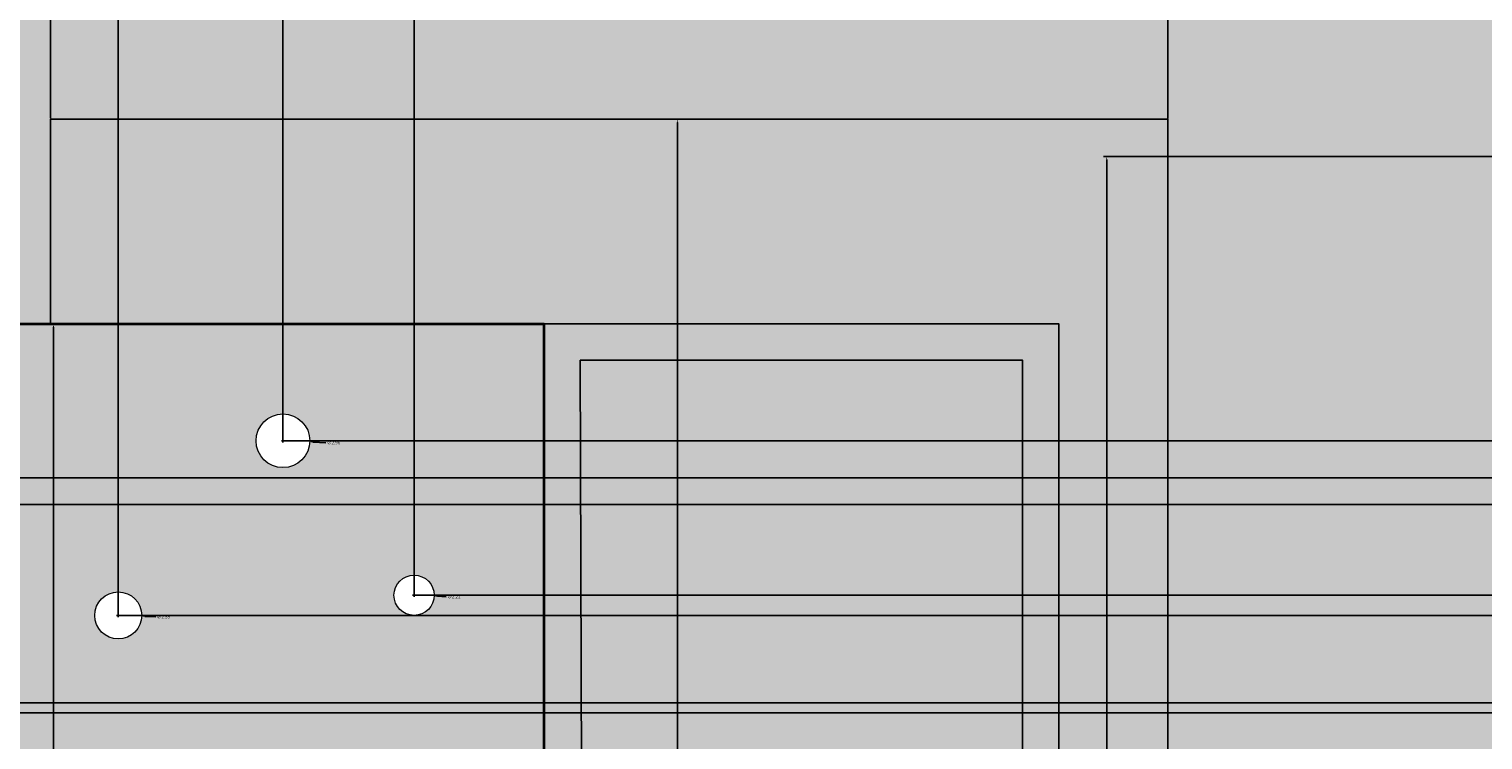
# Model space of a CAD drawing. Units: inches. Extents: x 73 to 607, y 92 to 651.
# Tile 5 of 18: x 368 to 448, y 224 to 264. Entities that reach past the tile are written whole.
import ezdxf

# ---------------------------------------------------------------- set-up
doc = ezdxf.new("R2010")
doc.units = ezdxf.units.IN
doc.header["$MEASUREMENT"] = 0
for name, color, linetype, lineweight in [('A-ANNO-DIMS', 2, 'Continuous', 18), ('A-ELEV', 7, 'Continuous', 35), ('A-ELEV-PANL', 7, 'Continuous', 18), ('A-ELEV-PATT-BKGD', 252, 'Continuous', 13), ('A-ELEV-PATT-FRAM', 38, 'Continuous', 13), ('A-ELEV-PATT-SHAD', 8, 'Continuous', 13), ('A-ELEV-PATT-WALL', 254, 'Continuous', 13), ('A-ELEV-PATT-WOOD', 32, 'Continuous', 13), ('A-GLAZ', 4, 'Continuous', 25), ('A-GLAZ-PATT', 7, 'Continuous', 13)]:
    doc.layers.add(name, color=color, linetype=linetype, lineweight=lineweight)
doc.styles.get("Standard").update_dxf_attribs({"font": 'arial.ttf'})
doc.dimstyles.get("Standard").update_dxf_attribs({"dimtxt": 0.18, "dimasz": 0.18, "dimexe": 0.18, "dimexo": 0.0625, "dimgap": 0.09, "dimtad": 0, "dimtih": 1, "dimtoh": 1, "dimdec": 4, "dimzin": 0, "dimdsep": 46, "dimtxsty": 'Standard', "dimcen": 0.09, "dimadec": 0, "dimazin": 0, "dimtfac": 1, "dimtdec": 4, "dimtofl": 0, "dimtmove": 0, "dimatfit": 3, "dimfxl": 1, "dimtolj": 1, "dimtzin": 0, "dimarcsym": 0})

# ---------------------------------------------------------------- blocks, each defined once
blk = doc.blocks.new('*D17')
at = {"layer": 'A-ANNO-DIMS', "color": 0, "lineweight": -2, "transparency": 16777216}
for p, q in [((580.161, 262.302), (607.278, 262.302)), ((607.098, 262.122), (607.098, 224.164)), ((607.098, 185.842), (607.098, 223.8)), ((431.133, 185.662), (607.278, 185.662))]:
    blk.add_line(p, q, dxfattribs=at)
at = {"layer": 'A-ANNO-DIMS', "color": 0, "transparency": 16777216}
for points in [[(607.068, 262.122), (607.128, 262.122), (607.098, 262.302)], [(607.068, 185.842), (607.128, 185.842), (607.098, 185.662)]]:
    blk.add_solid(points, dxfattribs=at)
at = {"layer": 'Defpoints', "color": 0, "transparency": 16777216}
for p in [(580.098, 262.302), (607.098, 262.302), (431.07, 185.662)]:
    blk.add_point(p, dxfattribs=at)
at = {"layer": 'A-ANNO-DIMS', "color": 0, "transparency": 16777216, "insert": (607.098, 223.982), "char_height": 0.18, "attachment_point": 5}
blk.add_mtext('\\A1;76.64', dxfattribs=at)
blk = doc.blocks.new('*D36')
at = {"layer": 'A-ANNO-DIMS', "color": 0, "lineweight": -2, "transparency": 16777216}
for p, q in [((396.63, 247.405), (369.512, 247.405)), ((369.692, 247.225), (369.692, 221.153)), ((369.692, 194.717), (369.692, 220.789)), ((396.63, 194.537), (369.512, 194.537))]:
    blk.add_line(p, q, dxfattribs=at)
at = {"layer": 'A-ANNO-DIMS', "color": 0, "transparency": 16777216}
for points in [[(369.662, 247.225), (369.722, 247.225), (369.692, 247.405)], [(369.662, 194.717), (369.722, 194.717), (369.692, 194.537)]]:
    blk.add_solid(points, dxfattribs=at)
at = {"layer": 'Defpoints', "color": 0, "transparency": 16777216}
for p in [(369.692, 247.405), (396.692, 247.405), (396.692, 194.537)]:
    blk.add_point(p, dxfattribs=at)
at = {"layer": 'A-ANNO-DIMS', "color": 0, "transparency": 16777216, "insert": (369.692, 220.971), "char_height": 0.18, "attachment_point": 5}
blk.add_mtext('\\A1;52.87', dxfattribs=at)
blk = doc.blocks.new('*D37')
at = {"layer": 'A-ANNO-DIMS', "color": 0, "lineweight": -2, "transparency": 16777216}
for p, q in [((369.534, 258.754), (369.534, 285.871)), ((369.714, 285.691), (399.908, 285.691)), ((430.89, 285.691), (400.696, 285.691)), ((431.07, 258.754), (431.07, 285.871))]:
    blk.add_line(p, q, dxfattribs=at)
at = {"layer": 'A-ANNO-DIMS', "color": 0, "transparency": 16777216}
for points in [[(369.714, 285.721), (369.714, 285.661), (369.534, 285.691)], [(430.89, 285.721), (430.89, 285.661), (431.07, 285.691)]]:
    blk.add_solid(points, dxfattribs=at)
at = {"layer": 'Defpoints', "color": 0, "transparency": 16777216}
for p in [(431.07, 285.691), (369.534, 258.691), (431.07, 258.691)]:
    blk.add_point(p, dxfattribs=at)
at = {"layer": 'A-ANNO-DIMS', "color": 0, "transparency": 16777216, "insert": (400.302, 285.691), "char_height": 0.18, "attachment_point": 5}
blk.add_mtext('\\A1;61.54', dxfattribs=at)
blk = doc.blocks.new('*D38')
at = {"layer": 'A-ANNO-DIMS', "color": 0, "lineweight": -2, "transparency": 16777216}
for p, q in [((431.008, 258.691), (403.89, 258.691)), ((404.07, 258.511), (404.07, 222.359)), ((404.07, 185.842), (404.07, 221.995)), ((431.008, 185.662), (403.89, 185.662))]:
    blk.add_line(p, q, dxfattribs=at)
at = {"layer": 'A-ANNO-DIMS', "color": 0, "transparency": 16777216}
for points in [[(404.04, 258.511), (404.1, 258.511), (404.07, 258.691)], [(404.04, 185.842), (404.1, 185.842), (404.07, 185.662)]]:
    blk.add_solid(points, dxfattribs=at)
at = {"layer": 'Defpoints', "color": 0, "transparency": 16777216}
for p in [(404.07, 258.691), (431.07, 258.691), (431.07, 185.662)]:
    blk.add_point(p, dxfattribs=at)
at = {"layer": 'A-ANNO-DIMS', "color": 0, "transparency": 16777216, "insert": (404.07, 222.177), "char_height": 0.18, "attachment_point": 5}
blk.add_mtext('\\A1;73.03', dxfattribs=at)
blk = doc.blocks.new('*D40')
at = {"layer": 'A-ANNO-DIMS', "color": 0, "lineweight": -2, "transparency": 16777216}
for p, q in [((454.642, 256.632), (427.525, 256.632)), ((427.705, 256.452), (427.705, 215.899)), ((427.705, 174.982), (427.705, 215.535)), ((454.642, 174.802), (427.525, 174.802))]:
    blk.add_line(p, q, dxfattribs=at)
at = {"layer": 'A-ANNO-DIMS', "color": 0, "transparency": 16777216}
for points in [[(427.675, 256.452), (427.735, 256.452), (427.705, 256.632)], [(427.675, 174.982), (427.735, 174.982), (427.705, 174.802)]]:
    blk.add_solid(points, dxfattribs=at)
at = {"layer": 'Defpoints', "color": 0, "transparency": 16777216}
for p in [(427.705, 256.632), (454.705, 256.632), (454.705, 174.802)]:
    blk.add_point(p, dxfattribs=at)
at = {"layer": 'A-ANNO-DIMS', "color": 0, "transparency": 16777216, "insert": (427.705, 215.717), "char_height": 0.18, "attachment_point": 5}
blk.add_mtext('\\A1;81.83', dxfattribs=at)
blk = doc.blocks.new('*D83')
at = {"layer": 'A-ANNO-DIMS', "color": 0, "lineweight": -2, "transparency": 16777216}
for p, q in [((360.849, 238.997), (360.849, 650.981)), ((361.029, 650.801), (366.597, 650.801)), ((373.077, 650.801), (367.508, 650.801)), ((373.257, 231.411), (373.257, 650.981))]:
    blk.add_line(p, q, dxfattribs=at)
at = {"layer": 'A-ANNO-DIMS', "color": 0, "transparency": 16777216}
for points in [[(361.029, 650.831), (361.029, 650.771), (360.849, 650.801)], [(373.077, 650.831), (373.077, 650.771), (373.257, 650.801)]]:
    blk.add_solid(points, dxfattribs=at)
at = {"layer": 'Defpoints', "color": 0, "transparency": 16777216}
for p in [(373.257, 650.801), (360.849, 238.935), (373.257, 231.348)]:
    blk.add_point(p, dxfattribs=at)
at = {"layer": 'A-ANNO-DIMS', "color": 0, "transparency": 16777216, "insert": (367.053, 650.801), "char_height": 0.18, "attachment_point": 5}
blk.add_mtext('\\A1;12.408', dxfattribs=at)
blk = doc.blocks.new('*D84')
at = {"layer": 'A-ANNO-DIMS', "color": 0, "lineweight": -2, "transparency": 16777216}
for p, q in [((373.257, 231.411), (373.257, 650.981)), ((373.437, 650.801), (377.4, 650.801)), ((382.151, 650.801), (378.187, 650.801)), ((382.331, 241.033), (382.331, 650.981))]:
    blk.add_line(p, q, dxfattribs=at)
at = {"layer": 'A-ANNO-DIMS', "color": 0, "transparency": 16777216}
for points in [[(373.437, 650.831), (373.437, 650.771), (373.257, 650.801)], [(382.151, 650.831), (382.151, 650.771), (382.331, 650.801)]]:
    blk.add_solid(points, dxfattribs=at)
at = {"layer": 'Defpoints', "color": 0, "transparency": 16777216}
for p in [(382.331, 650.801), (382.331, 240.97), (373.257, 231.348)]:
    blk.add_point(p, dxfattribs=at)
at = {"layer": 'A-ANNO-DIMS', "color": 0, "transparency": 16777216, "insert": (377.794, 650.801), "char_height": 0.18, "attachment_point": 5}
blk.add_mtext('\\A1;9.074', dxfattribs=at)
blk = doc.blocks.new('*D85')
at = {"layer": 'A-ANNO-DIMS', "color": 0, "lineweight": -2, "transparency": 16777216}
for p, q in [((382.331, 241.033), (382.331, 650.981)), ((382.511, 650.801), (385.55, 650.801)), ((389.373, 650.801), (386.334, 650.801)), ((389.553, 232.521), (389.553, 650.981))]:
    blk.add_line(p, q, dxfattribs=at)
at = {"layer": 'A-ANNO-DIMS', "color": 0, "transparency": 16777216}
for points in [[(382.511, 650.831), (382.511, 650.771), (382.331, 650.801)], [(389.373, 650.831), (389.373, 650.771), (389.553, 650.801)]]:
    blk.add_solid(points, dxfattribs=at)
at = {"layer": 'Defpoints', "color": 0, "transparency": 16777216}
for p in [(389.553, 650.801), (382.331, 240.97), (389.553, 232.458)]:
    blk.add_point(p, dxfattribs=at)
at = {"layer": 'A-ANNO-DIMS', "color": 0, "transparency": 16777216, "insert": (385.942, 650.801), "char_height": 0.18, "attachment_point": 5}
blk.add_mtext('\\A1;7.222', dxfattribs=at)
blk = doc.blocks.new('*D93')
at = {"layer": 'A-ANNO-DIMS', "color": 0, "lineweight": -2, "transparency": 16777216}
for p, q in [((349.059, 237.455), (607.278, 237.455)), ((607.098, 237.275), (607.098, 232.178)), ((607.098, 226.717), (607.098, 231.814)), ((349.059, 226.537), (607.278, 226.537))]:
    blk.add_line(p, q, dxfattribs=at)
at = {"layer": 'A-ANNO-DIMS', "color": 0, "transparency": 16777216}
for points in [[(607.068, 237.275), (607.128, 237.275), (607.098, 237.455)], [(607.068, 226.717), (607.128, 226.717), (607.098, 226.537)]]:
    blk.add_solid(points, dxfattribs=at)
at = {"layer": 'Defpoints', "color": 0, "transparency": 16777216}
for p in [(348.997, 237.455), (348.997, 226.537), (607.098, 226.537)]:
    blk.add_point(p, dxfattribs=at)
at = {"layer": 'A-ANNO-DIMS', "color": 0, "transparency": 16777216, "insert": (607.098, 231.996), "char_height": 0.18, "attachment_point": 5}
blk.add_mtext('\\A1;10.917', dxfattribs=at)
blk = doc.blocks.new('*D95')
at = {"layer": 'A-ANNO-DIMS', "color": 0, "lineweight": -2, "transparency": 16777216}
for p, q in [((363.874, 225.982), (607.278, 225.982)), ((607.098, 225.802), (607.098, 212.749)), ((607.098, 199.331), (607.098, 212.385)), ((363.319, 199.151), (607.278, 199.151))]:
    blk.add_line(p, q, dxfattribs=at)
at = {"layer": 'A-ANNO-DIMS', "color": 0, "transparency": 16777216}
for points in [[(607.068, 225.802), (607.128, 225.802), (607.098, 225.982)], [(607.068, 199.331), (607.128, 199.331), (607.098, 199.151)]]:
    blk.add_solid(points, dxfattribs=at)
at = {"layer": 'Defpoints', "color": 0, "transparency": 16777216}
for p in [(363.812, 225.982), (607.098, 225.982), (363.256, 199.151)]:
    blk.add_point(p, dxfattribs=at)
at = {"layer": 'A-ANNO-DIMS', "color": 0, "transparency": 16777216, "insert": (607.098, 212.567), "char_height": 0.18, "attachment_point": 5}
blk.add_mtext('\\A1;26.83', dxfattribs=at)
blk = doc.blocks.new('*D96')
at = {"layer": 'A-ANNO-DIMS', "color": 0, "lineweight": -2, "transparency": 16777216}
for p, q in [((360.911, 238.935), (607.278, 238.935)), ((607.098, 238.755), (607.098, 232.64)), ((607.098, 226.162), (607.098, 232.276)), ((363.874, 225.982), (607.278, 225.982))]:
    blk.add_line(p, q, dxfattribs=at)
at = {"layer": 'A-ANNO-DIMS', "color": 0, "transparency": 16777216}
for points in [[(607.068, 238.755), (607.128, 238.755), (607.098, 238.935)], [(607.068, 226.162), (607.128, 226.162), (607.098, 225.982)]]:
    blk.add_solid(points, dxfattribs=at)
at = {"layer": 'Defpoints', "color": 0, "transparency": 16777216}
for p in [(360.849, 238.935), (607.098, 238.935), (363.812, 225.982)]:
    blk.add_point(p, dxfattribs=at)
at = {"layer": 'A-ANNO-DIMS', "color": 0, "transparency": 16777216, "insert": (607.098, 232.458), "char_height": 0.18, "attachment_point": 5}
blk.add_mtext('\\A1;12.953', dxfattribs=at)
blk = doc.blocks.new('*D99')
at = {"layer": 'A-ANNO-DIMS', "color": 0, "lineweight": -2, "transparency": 16777216}
for p, q in [((373.319, 231.348), (607.278, 231.348)), ((607.098, 231.168), (607.098, 220.428)), ((607.098, 209.323), (607.098, 220.064)), ((377.023, 209.143), (607.278, 209.143))]:
    blk.add_line(p, q, dxfattribs=at)
at = {"layer": 'A-ANNO-DIMS', "color": 0, "transparency": 16777216}
for points in [[(607.068, 231.168), (607.128, 231.168), (607.098, 231.348)], [(607.068, 209.323), (607.128, 209.323), (607.098, 209.143)]]:
    blk.add_solid(points, dxfattribs=at)
at = {"layer": 'Defpoints', "color": 0, "transparency": 16777216}
for p in [(373.257, 231.348), (607.098, 231.348), (376.96, 209.143)]:
    blk.add_point(p, dxfattribs=at)
at = {"layer": 'A-ANNO-DIMS', "color": 0, "transparency": 16777216, "insert": (607.098, 220.246), "char_height": 0.18, "attachment_point": 5}
blk.add_mtext('\\A1;22.205', dxfattribs=at)
blk = doc.blocks.new('*D101')
at = {"layer": 'A-ANNO-DIMS', "color": 0, "lineweight": -2, "transparency": 16777216}
for p, q in [((382.393, 240.97), (607.278, 240.97)), ((607.098, 240.79), (607.098, 231.715)), ((607.098, 222.276), (607.098, 231.351)), ((382.949, 222.096), (607.278, 222.096))]:
    blk.add_line(p, q, dxfattribs=at)
at = {"layer": 'A-ANNO-DIMS', "color": 0, "transparency": 16777216}
for points in [[(607.068, 240.79), (607.128, 240.79), (607.098, 240.97)], [(607.068, 222.276), (607.128, 222.276), (607.098, 222.096)]]:
    blk.add_solid(points, dxfattribs=at)
at = {"layer": 'Defpoints', "color": 0, "transparency": 16777216}
for p in [(382.331, 240.97), (607.098, 240.97), (382.886, 222.096)]:
    blk.add_point(p, dxfattribs=at)
at = {"layer": 'A-ANNO-DIMS', "color": 0, "transparency": 16777216, "insert": (607.098, 231.533), "char_height": 0.18, "attachment_point": 5}
blk.add_mtext('\\A1;18.874', dxfattribs=at)
blk = doc.blocks.new('*D102')
at = {"layer": 'A-ANNO-DIMS', "color": 0, "lineweight": -2, "transparency": 16777216}
for p, q in [((382.393, 240.97), (607.278, 240.97)), ((607.098, 240.79), (607.098, 236.896)), ((607.098, 232.638), (607.098, 236.532)), ((389.616, 232.458), (607.278, 232.458))]:
    blk.add_line(p, q, dxfattribs=at)
at = {"layer": 'A-ANNO-DIMS', "color": 0, "transparency": 16777216}
for points in [[(607.068, 240.79), (607.128, 240.79), (607.098, 240.97)], [(607.068, 232.638), (607.128, 232.638), (607.098, 232.458)]]:
    blk.add_solid(points, dxfattribs=at)
at = {"layer": 'Defpoints', "color": 0, "transparency": 16777216}
for p in [(382.331, 240.97), (389.553, 232.458), (607.098, 232.458)]:
    blk.add_point(p, dxfattribs=at)
at = {"layer": 'A-ANNO-DIMS', "color": 0, "transparency": 16777216, "insert": (607.098, 236.714), "char_height": 0.18, "attachment_point": 5}
blk.add_mtext('\\A1;8.512', dxfattribs=at)
blk = doc.blocks.new('*D144')
at = {"layer": 'A-ANNO-DIMS', "color": 0, "lineweight": -2, "transparency": 16777216}
for p, q in [((382.331, 240.88), (382.331, 241.06)), ((382.241, 240.97), (382.421, 240.97)), ((384.697, 240.864), (383.989, 240.896))]:
    blk.add_line(p, q, dxfattribs=at)
at = {"layer": 'A-ANNO-DIMS', "color": 0, "transparency": 16777216}
blk.add_solid([(383.991, 240.925), (383.988, 240.866), (383.81, 240.904)], dxfattribs=at)
at = {"layer": 'Defpoints', "color": 0, "transparency": 16777216}
for p in [(380.852, 241.037), (383.81, 240.904)]:
    blk.add_point(p, dxfattribs=at)
at = {"layer": 'A-ANNO-DIMS', "color": 0, "transparency": 16777216, "insert": (385.119, 240.864), "char_height": 0.18, "attachment_point": 5}
blk.add_mtext('\\A1;∅2.96', dxfattribs=at)
blk = doc.blocks.new('*D145')
at = {"layer": 'A-ANNO-DIMS', "color": 0, "lineweight": -2, "transparency": 16777216}
for p, q in [((373.257, 231.258), (373.257, 231.438)), ((373.167, 231.348), (373.347, 231.348)), ((375.328, 231.273), (374.731, 231.295))]:
    blk.add_line(p, q, dxfattribs=at)
at = {"layer": 'A-ANNO-DIMS', "color": 0, "transparency": 16777216}
blk.add_solid([(374.732, 231.325), (374.73, 231.265), (374.551, 231.301)], dxfattribs=at)
at = {"layer": 'Defpoints', "color": 0, "transparency": 16777216}
for p in [(371.962, 231.395), (374.551, 231.301)]:
    blk.add_point(p, dxfattribs=at)
at = {"layer": 'A-ANNO-DIMS', "color": 0, "transparency": 16777216, "insert": (375.75, 231.273), "char_height": 0.18, "attachment_point": 5}
blk.add_mtext('\\A1;∅2.59', dxfattribs=at)
blk = doc.blocks.new('*D146')
at = {"layer": 'A-ANNO-DIMS', "color": 0, "lineweight": -2, "transparency": 16777216}
for p, q in [((389.463, 232.458), (389.643, 232.458)), ((389.553, 232.368), (389.553, 232.548)), ((391.328, 232.376), (390.842, 232.399))]:
    blk.add_line(p, q, dxfattribs=at)
at = {"layer": 'A-ANNO-DIMS', "color": 0, "transparency": 16777216}
blk.add_solid([(390.843, 232.428), (390.841, 232.369), (390.662, 232.407)], dxfattribs=at)
at = {"layer": 'Defpoints', "color": 0, "transparency": 16777216}
for p in [(388.444, 232.51), (390.662, 232.407)]:
    blk.add_point(p, dxfattribs=at)
at = {"layer": 'A-ANNO-DIMS', "color": 0, "transparency": 16777216, "insert": (391.748, 232.376), "char_height": 0.18, "attachment_point": 5}
blk.add_mtext('\\A1;∅2.22', dxfattribs=at)

msp = doc.modelspace()

# ---------------------------------------------------------------- hatches: boundary and pattern name
at = {"layer": 'A-ELEV-PATT-BKGD'}
h = msp.add_hatch(color=256, dxfattribs=at)
h.dxf.hatch_style = 1
h.paths.add_polyline_path([(321.3008, 479.2042), (312.3008, 479.2042), (312.3008, 478.7576), (312.3008, 412.636), (321.3008, 412.636)])
h.paths.add_polyline_path([(312.3008, 504.7576), (256.4726, 504.7576), (256.4726, 503.4576), (312.3008, 503.4576)], flags=17)
h.paths.add_polyline_path([(321.3008, 543.1576), (321.3008, 552.1576), (320.3257, 552.1576), (312.3008, 552.1576), (256.4726, 552.1576), (256.4726, 543.1576), (312.3008, 543.1576), (312.3008, 479.2042), (321.3008, 479.2042)])
h.paths.add_polyline_path([(451.5214, 412.636), (256.4726, 412.636), (256.4726, 403.636), (442.5214, 403.636), (442.5214, 320.2042), (206.1343, 320.2042), (206.1343, 320.9135), (206.1343, 403.636), (256.4726, 403.636), (256.4726, 412.636), (201.6343, 412.636), (201.6343, 320.9135), (201.6343, 320.2042), (201.6343, 311.2042), (256.4726, 311.2042), (451.5214, 311.2042)])
h.paths.add_polyline_path([(431.07, 258.6914), (369.5339, 258.6914), (369.5339, 247.4054), (396.692, 247.4054), (425.07, 247.4054), (425.07, 194.7312), (396.692, 194.6197), (396.692, 194.5366), (369.5339, 194.5366), (369.5339, 185.6619), (431.07, 185.6619)])
h.paths.add_polyline_path([(580.0983, 262.3024), (451.5214, 262.3024), (451.5214, 143.2042), (580.0983, 143.2042)])
h.paths.add_polyline_path([(454.7049, 174.802), (454.7049, 256.6321), (577.9249, 256.6321), (577.9249, 174.802)], flags=16)
h.paths.add_polyline_path([(465.9716, 191.1416, -1), (473.7874, 191.1416, -1)], flags=0)
h.paths.add_polyline_path([(490.5373, 181.6586, -1), (494.9999, 181.6586, -1)], flags=0)
h.paths.add_polyline_path([(476.2996, 209.8287, -1), (500.5844, 209.8287, -1)], flags=0)
h.paths.add_polyline_path([(505.3326, 194.7675, -1), (512.5843, 194.7675, -1)], flags=0)
h.paths.add_polyline_path([(520.9613, 186.679, -1), (526.544, 186.679, -1)], flags=0)
h.paths.add_polyline_path([(466.8103, 225.7267, -1), (470.1573, 225.7267, -1)], flags=0)
h.paths.add_polyline_path([(527.1059, 203.6926, -1), (536.0311, 203.6926, -1)], flags=0)
h.paths.add_polyline_path([(504.775, 232.6995, -1), (513.7002, 232.6995, -1)], flags=0)
h.paths.add_polyline_path([(546.9241, 183.611, -1), (554.7336, 183.611, -1)], flags=0)
h.paths.add_polyline_path([(459.5544, 243.856, -1), (466.8061, 243.856, -1)], flags=0)
h.paths.add_polyline_path([(476.3045, 246.924, -1), (488.5767, 246.924, -1)], flags=0)
h.paths.add_polyline_path([(529.9044, 226.8424, -1), (556.68, 226.8424, -1)], flags=0)
h.paths.add_polyline_path([(554.1814, 203.9716, -1), (561.4331, 203.9716, -1)], flags=0)
h.paths.add_polyline_path([(567.8561, 193.3729, -1), (570.6475, 193.3729, -1)], flags=0)
h.paths.add_polyline_path([(522.3584, 250.271, -1), (525.7053, 250.271, -1)], flags=0)
h.paths.add_polyline_path([(561.9965, 245.2506, -1), (567.5748, 245.2506, -1)], flags=0)
h.paths.add_polyline_path([(347.8686, 194.5366), (341.8686, 194.5366), (341.8686, 194.5452), (314.0144, 194.5452), (314.0144, 188.5452), (347.8686, 188.5452)])
h.paths.add_polyline_path([(347.8686, 253.4054), (314.0144, 253.4054), (314.0144, 247.4054), (341.8686, 247.4054), (347.8686, 247.4054)])
h.paths.add_polyline_path([(304.3559, 253.4054), (298.3559, 253.4054), (298.3559, 188.5452), (304.3559, 188.5452)])
h.paths.add_polyline_path([(450.6603, 552.1576), (369.9727, 552.1576), (369.9727, 479.2042), (374.4727, 479.2042), (374.4727, 547.6576), (446.1603, 547.6576), (446.1603, 479.2042), (450.6603, 479.2042)])
h.paths.add_polyline_path([(374.4727, 479.2042), (369.9727, 479.2042), (369.9727, 465.0632), (374.4727, 465.0632)])
h.paths.add_polyline_path([(450.6603, 479.2042), (446.1603, 479.2042), (446.1603, 465.0632), (450.6603, 465.0632)])
h.paths.add_polyline_path([(256.4726, 281.6039), (109.0983, 281.6039), (100.0983, 281.6039), (100.0983, 167.2042), (100.0983, 143.2042), (109.0983, 143.2042), (109.0983, 167.2042), (109.0983, 272.6039), (256.4726, 272.6039)])
at = {"layer": 'A-ELEV-PATT-FRAM'}
h = msp.add_hatch(color=256, dxfattribs=at)
h.dxf.hatch_style = 1
h.paths.add_polyline_path([(433.025, 403.636), (409.515, 403.636), (409.515, 342.1009), (411.515, 342.1009), (411.515, 401.636), (431.025, 401.636), (431.025, 342.1009), (433.025, 342.1009)])
h.paths.add_polyline_path([(433.025, 341.1009), (431.025, 341.1009), (431.025, 340.0025), (411.515, 340.0025), (411.515, 341.1009), (409.515, 341.1009), (409.515, 338.0025), (433.025, 338.0025)])
h.paths.add_polyline_path([(425.07, 247.4054), (396.692, 247.4054), (396.692, 194.6197), (425.07, 194.7312)])
h.paths.add_polyline_path([(423.07, 245.4054), (423.07, 196.7234), (398.8836, 196.6284), (398.692, 245.4054)], flags=16)
h.paths.add_polyline_path([(341.8686, 247.4054), (314.0144, 247.4054), (314.0144, 245.4054), (339.8686, 245.4054), (339.8686, 196.5452), (314.0144, 196.5452), (314.0144, 194.5452), (341.8686, 194.5452)])
h.paths.add_polyline_path([(372.3213, 383.1812), (350.3213, 383.1812), (350.3213, 342.1009), (372.3213, 342.1009)], flags=16)
h.paths.add_polyline_path([(376.3213, 389.1812), (346.3213, 389.1812), (346.3213, 342.1009), (350.3213, 342.1009), (350.3213, 383.1812), (372.3213, 383.1812), (372.3213, 342.1009), (376.3213, 342.1009)], flags=17)
h.paths.add_polyline_path([(375.3213, 362.2042, -1), (373.3213, 362.2042, -1)], flags=16)
h.paths.add_polyline_path([(379.3213, 392.2042), (343.3213, 392.2042), (343.3213, 342.1009), (346.3213, 342.1009), (346.3213, 389.1812), (376.3213, 389.1812), (376.3213, 342.1009), (379.3213, 342.1009)])
h.paths.add_polyline_path([(350.3213, 341.1009), (346.3213, 341.1009), (346.3213, 338.0025), (350.3213, 338.0025)])
h.paths.add_polyline_path([(346.3213, 341.1009), (343.3213, 341.1009), (343.3213, 338.0025), (346.3213, 338.0025)])
h.paths.add_polyline_path([(346.3213, 337.0025), (343.3213, 337.0025), (343.3213, 332.9397), (346.3213, 332.9397)])
h.paths.add_polyline_path([(350.3213, 337.0025), (346.3213, 337.0025), (346.3213, 332.9397), (350.3213, 332.9397)])
h.paths.add_polyline_path([(350.3213, 331.9397), (346.3213, 331.9397), (346.3213, 320.2042), (376.3213, 320.2042), (376.3213, 331.9397), (372.3213, 331.9397), (372.3213, 326.2042), (350.3213, 326.2042)])
h.paths.add_polyline_path([(372.3213, 337.0025), (350.3213, 337.0025), (350.3213, 332.9397), (372.3213, 332.9397)])
h.paths.add_polyline_path([(372.3213, 341.1009), (350.3213, 341.1009), (350.3213, 338.0025), (372.3213, 338.0025)])
h.paths.add_polyline_path([(376.3213, 341.1009), (372.3213, 341.1009), (372.3213, 338.0025), (376.3213, 338.0025)])
h.paths.add_polyline_path([(376.3213, 337.0025), (372.3213, 337.0025), (372.3213, 332.9397), (376.3213, 332.9397)])
h.paths.add_polyline_path([(379.3213, 341.1009), (376.3213, 341.1009), (376.3213, 338.0025), (379.3213, 338.0025)])
h.paths.add_polyline_path([(379.3213, 337.0025), (376.3213, 337.0025), (376.3213, 332.9397), (379.3213, 332.9397)])
h.paths.add_polyline_path([(379.3213, 331.9397), (376.3213, 331.9397), (376.3213, 320.2042), (379.3213, 320.2042)])
h.paths.add_polyline_path([(372.3213, 331.9397), (350.3213, 331.9397), (350.3213, 326.2042), (372.3213, 326.2042)], flags=17)
h.paths.add_polyline_path([(346.3213, 331.9397), (343.3213, 331.9397), (343.3213, 320.2042), (346.3213, 320.2042)])
at = {"layer": 'A-ELEV-PATT-SHAD'}
h = msp.add_hatch(color=256, dxfattribs=at)
h.dxf.hatch_style = 1
h.paths.add_polyline_path([(451.5214, 412.636), (256.4726, 412.636), (256.4726, 403.636), (442.5214, 403.636), (442.5214, 320.2042), (206.1343, 320.2042), (206.1343, 320.9135), (206.1343, 403.636), (256.4726, 403.636), (256.4726, 412.636), (201.6343, 412.636), (201.6343, 320.9135), (201.6343, 320.2042), (201.6343, 311.2042), (256.4726, 311.2042), (451.5214, 311.2042)])
h.paths.add_polyline_path([(580.0983, 262.3024), (451.5214, 262.3024), (451.5214, 143.2042), (580.0983, 143.2042)])
h.paths.add_polyline_path([(454.7049, 174.802), (454.7049, 256.6321), (577.9249, 256.6321), (577.9249, 174.802)], flags=16)
h.paths.add_polyline_path([(465.9716, 191.1416, -1), (473.7874, 191.1416, -1)], flags=0)
h.paths.add_polyline_path([(490.5373, 181.6586, -1), (494.9999, 181.6586, -1)], flags=0)
h.paths.add_polyline_path([(476.2996, 209.8287, -1), (500.5844, 209.8287, -1)], flags=0)
h.paths.add_polyline_path([(505.3326, 194.7675, -1), (512.5843, 194.7675, -1)], flags=0)
h.paths.add_polyline_path([(520.9613, 186.679, -1), (526.544, 186.679, -1)], flags=0)
h.paths.add_polyline_path([(466.8103, 225.7267, -1), (470.1573, 225.7267, -1)], flags=0)
h.paths.add_polyline_path([(527.1059, 203.6926, -1), (536.0311, 203.6926, -1)], flags=0)
h.paths.add_polyline_path([(459.5544, 243.856, -1), (466.8061, 243.856, -1)], flags=0)
h.paths.add_polyline_path([(504.775, 232.6995, -1), (513.7002, 232.6995, -1)], flags=0)
h.paths.add_polyline_path([(476.3045, 246.924, -1), (488.5767, 246.924, -1)], flags=0)
h.paths.add_polyline_path([(546.9241, 183.611, -1), (554.7336, 183.611, -1)], flags=0)
h.paths.add_polyline_path([(529.9044, 226.8424, -1), (556.68, 226.8424, -1)], flags=0)
h.paths.add_polyline_path([(554.1814, 203.9716, -1), (561.4331, 203.9716, -1)], flags=0)
h.paths.add_polyline_path([(522.3584, 250.271, -1), (525.7053, 250.271, -1)], flags=0)
h.paths.add_polyline_path([(567.8561, 193.3729, -1), (570.6475, 193.3729, -1)], flags=0)
h.paths.add_polyline_path([(561.9965, 245.2506, -1), (567.5748, 245.2506, -1)], flags=0)
h.paths.add_polyline_path([(431.07, 258.6914), (369.5339, 258.6914), (369.5339, 247.4054), (396.692, 247.4054), (425.07, 247.4054), (425.07, 194.7312), (396.692, 194.6197), (396.692, 194.5366), (369.5339, 194.5366), (369.5339, 185.6619), (431.07, 185.6619)])
h.paths.add_polyline_path([(347.8686, 253.4054), (314.0144, 253.4054), (314.0144, 247.4054), (341.8686, 247.4054), (347.8686, 247.4054)])
h.paths.add_polyline_path([(304.3559, 253.4054), (298.3559, 253.4054), (298.3559, 188.5452), (304.3559, 188.5452)])
h.paths.add_polyline_path([(347.8686, 194.5366), (341.8686, 194.5366), (341.8686, 194.5452), (314.0144, 194.5452), (314.0144, 188.5452), (347.8686, 188.5452)])
at = {"layer": 'A-ELEV-PATT-WALL'}
h = msp.add_hatch(color=256, dxfattribs=at)
h.dxf.hatch_style = 1
h.paths.add_polyline_path([(509.9692, 483.857), (450.6603, 483.857), (450.6603, 465.0632), (446.1603, 465.0632), (446.1603, 484.2142), (374.4727, 484.2142), (374.4727, 465.0632), (369.9727, 465.0632), (369.9727, 484.2142), (321.3008, 484.2142), (321.3008, 412.636), (451.5214, 412.636), (451.5214, 311.2042), (314.0144, 311.2042), (314.0144, 253.4054), (347.8686, 253.4054), (347.8686, 247.4054), (369.5339, 247.4054), (369.5339, 258.6914), (431.07, 258.6914), (431.07, 185.6619), (369.5339, 185.6619), (369.5339, 194.5366), (347.8686, 194.5366), (347.8686, 188.5452), (314.0144, 188.5452), (314.0144, 143.2042), (451.5214, 143.2042), (451.5214, 262.3024), (580.0983, 262.3024), (580.0983, 311.2042), (509.9692, 311.2042)])
h.paths.add_polyline_path([(304.3559, 311.2042), (256.4726, 311.2042), (256.4726, 167.2042), (256.4726, 143.2042), (304.3559, 143.2042), (304.3559, 188.5452), (298.3559, 188.5452), (298.3559, 253.4054), (304.3559, 253.4054)])
at = {"layer": 'A-ELEV-PATT-WOOD'}
h = msp.add_hatch(color=256, dxfattribs=at)
h.dxf.hatch_style = 1
h.paths.add_polyline_path([(396.692, 247.4054), (341.8686, 247.4054), (341.8686, 194.5366), (375.5339, 194.5366), (396.692, 194.6197)])
h.paths.add_polyline_path([(390.6634, 232.4585, -1), (388.443, 232.4585, -1)], flags=16)
h.paths.add_polyline_path([(384.3667, 222.0962, -1), (381.4061, 222.0962, -1)], flags=16)
h.paths.add_polyline_path([(380.8505, 240.9703, -1), (383.8112, 240.9703, -1)], flags=16)
h.paths.add_polyline_path([(371.9613, 231.3482, -1), (374.5519, 231.3482, -1)], flags=16)
h.paths.add_polyline_path([(363.0718, 225.982, -1), (364.5521, 225.982, -1)], flags=16)
h.paths.add_polyline_path([(379.1808, 209.1433, -1), (374.7399, 209.1433, -1)], flags=16)
h.paths.add_polyline_path([(357.8883, 238.9349, -1), (363.8096, 238.9349, -1)], flags=16)
h.paths.add_polyline_path([(362.6961, 213.0292, -1), (350.8535, 213.0292, -1)], flags=16)
h.paths.add_polyline_path([(388.8114, 200.0764, -1), (386.2208, 200.0764, -1)], flags=16)
h.paths.add_polyline_path([(352.6976, 226.5372, -1), (345.296, 226.5372, -1)], flags=16)
h.paths.add_polyline_path([(347.3301, 237.4546, -1), (350.6635, 237.4546, -1)], flags=16)
h.paths.add_polyline_path([(363.9971, 199.1512, -1), (362.5156, 199.1512, -1)], flags=16)
at = {"layer": 'A-GLAZ-PATT'}
h = msp.add_hatch(color=256, dxfattribs=at)
h.dxf.hatch_style = 1
h.set_gradient(color1=(0, 0, 255))
h.paths.add_polyline_path([(423.07, 245.4054), (398.692, 245.4054), (398.8836, 196.6284), (423.07, 196.7234)])

# ---------------------------------------------------------------- linework, layer by layer
at = {"layer": 'A-ELEV'}
msp.add_lwpolyline([(341.8686, 247.4054), (396.692, 247.4054), (396.692, 194.5366), (341.8686, 194.5366)], close=True, dxfattribs=at)
at = {"layer": 'A-ELEV-PANL'}
for centre, radius in [((382.3308, 240.9703), 1.4803), ((389.5532, 232.4585), 1.1102), ((373.2566, 231.3482), 1.2953)]:
    msp.add_circle(centre, radius, dxfattribs=at)
at = {"layer": 'A-GLAZ'}
msp.add_line((398.692, 245.4054), (398.8836, 196.6284), dxfattribs=at)
for points in [[(369.5339, 247.4054), (369.5339, 258.6914), (431.07, 258.6914), (431.07, 185.6619), (369.5339, 185.6619), (369.5339, 194.5366)], [(375.5339, 247.4054), (425.07, 247.4054), (425.07, 194.7312), (375.5339, 194.5366)], [(398.692, 245.4054), (423.07, 245.4054), (423.07, 196.7234), (398.8836, 196.6284)]]:
    msp.add_lwpolyline(points, dxfattribs=at)

# ---------------------------------------------------------------- dimensions: what is measured, and where the dimension line sits
at = {"layer": 'A-ANNO-DIMS'}
for base, p1, p2, override, picture, middle in [((373.2566, 650.801), (360.8489, 238.9349), (373.2566, 231.3482), {"dimdec": 3, "dimlfac": 1, "dimrnd": 0, "dimzin": 0, "dimdsep": 46, "dimlunit": 2}, '*D83', (367.0527, 650.801)), ((382.3308, 650.801), (373.2566, 231.3482), (382.3308, 240.9703), {"dimdec": 3, "dimlfac": 1, "dimrnd": 0, "dimzin": 0, "dimdsep": 46, "dimlunit": 2}, '*D84', (377.7937, 650.801)), ((389.5532, 650.801), (382.3308, 240.9703), (389.5532, 232.4585), {"dimdec": 3, "dimlfac": 1, "dimrnd": 0, "dimzin": 0, "dimdsep": 46, "dimlunit": 2}, '*D85', (385.942, 650.801)), ((431.07, 285.6914), (369.5339, 258.6914), (431.07, 258.6914), {"dimdec": 2, "dimlfac": 1, "dimrnd": 0, "dimzin": 0, "dimdsep": 46, "dimlunit": 2}, '*D37', (400.302, 285.6914))]:
    dim = msp.add_linear_dim(base=base, p1=p1, p2=p2, dimstyle='Standard', override=override, dxfattribs=at)
    dim.commit()
    dim.dimension.update_dxf_attribs({"geometry": picture, "text_midpoint": middle})
for base, p1, p2, override, picture, middle in [((607.0983, 262.3024), (431.07, 185.6619), (580.0983, 262.3024), {"dimdec": 2, "dimlfac": 1, "dimrnd": 0, "dimzin": 0, "dimdsep": 46, "dimlunit": 2}, '*D17', (607.0983, 223.9821)), ((404.07, 258.6914), (431.07, 185.6619), (431.07, 258.6914), {"dimdec": 2, "dimlfac": 1, "dimrnd": 0, "dimzin": 0, "dimdsep": 46, "dimlunit": 2}, '*D38', (404.07, 222.1767)), ((427.7049, 256.6321), (454.7049, 174.802), (454.7049, 256.6321), {"dimdec": 2, "dimlfac": 1, "dimrnd": 0, "dimzin": 0, "dimdsep": 46, "dimlunit": 2}, '*D40', (427.7049, 215.7171)), ((369.692, 247.4054), (396.692, 194.5366), (396.692, 247.4054), {"dimdec": 2, "dimlfac": 1, "dimrnd": 0, "dimzin": 0, "dimdsep": 46, "dimlunit": 2}, '*D36', (369.692, 220.971)), ((607.0983, 240.9703), (382.8864, 222.0962), (382.3308, 240.9703), {"dimdec": 3, "dimlfac": 1, "dimrnd": 0, "dimzin": 0, "dimdsep": 46, "dimlunit": 2}, '*D101', (607.0983, 231.5333)), ((607.0983, 232.4585), (382.3308, 240.9703), (389.5532, 232.4585), {"dimdec": 3, "dimlfac": 1, "dimrnd": 0, "dimzin": 0, "dimdsep": 46, "dimlunit": 2}, '*D102', (607.0983, 236.7144)), ((607.0983, 238.9349), (363.8119, 225.982), (360.8489, 238.9349), {"dimdec": 3, "dimlfac": 1, "dimrnd": 0, "dimzin": 0, "dimdsep": 46, "dimlunit": 2}, '*D96', (607.0983, 232.4585)), ((607.0983, 226.5372), (348.9968, 237.4546), (348.9968, 226.5372), {"dimdec": 3, "dimlfac": 1, "dimrnd": 0, "dimzin": 0, "dimdsep": 46, "dimlunit": 2}, '*D93', (607.0983, 231.9959)), ((607.0983, 231.3482), (376.9603, 209.1433), (373.2566, 231.3482), {"dimdec": 3, "dimlfac": 1, "dimrnd": 0, "dimzin": 0, "dimdsep": 46, "dimlunit": 2}, '*D99', (607.0983, 220.2458)), ((607.0983, 225.982), (363.2564, 199.1512), (363.8119, 225.982), {"dimdec": 2, "dimlfac": 1, "dimrnd": 0, "dimzin": 0, "dimdsep": 46, "dimlunit": 2}, '*D95', (607.0983, 212.5666))]:
    dim = msp.add_linear_dim(base=base, p1=p1, p2=p2, angle=90, dimstyle='Standard', override=override, dxfattribs=at)
    dim.commit()
    dim.dimension.update_dxf_attribs({"geometry": picture, "text_midpoint": middle})
for p1, p2, picture, middle in [((380.852, 241.037), (383.8096, 240.9036), '*D144', (384.6969, 240.8636)), ((388.4442, 232.51), (390.6622, 232.4069), '*D146', (391.3277, 232.3759)), ((371.9621, 231.395), (374.551, 231.3014), '*D145', (375.3277, 231.2733))]:
    dim = msp.add_diameter_dim_2p(p1=p1, p2=p2, dimstyle='Standard', override={"dimdec": 2, "dimlfac": 1, "dimrnd": 0, "dimzin": 0, "dimdsep": 46, "dimlunit": 2}, dxfattribs=at)
    dim.commit()
    dim.dimension.update_dxf_attribs({"geometry": picture, "text_midpoint": middle, "dimtype": 163})

doc.saveas('drawing.dxf')
